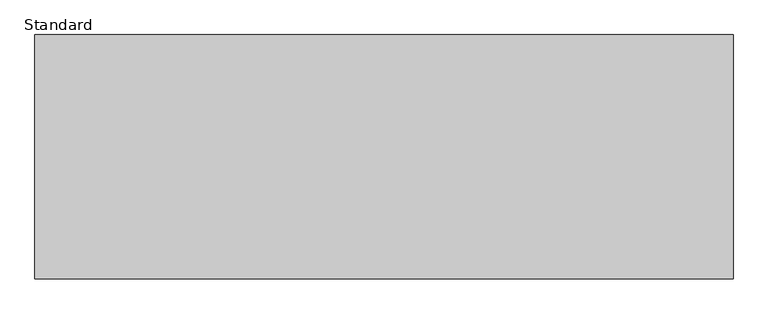
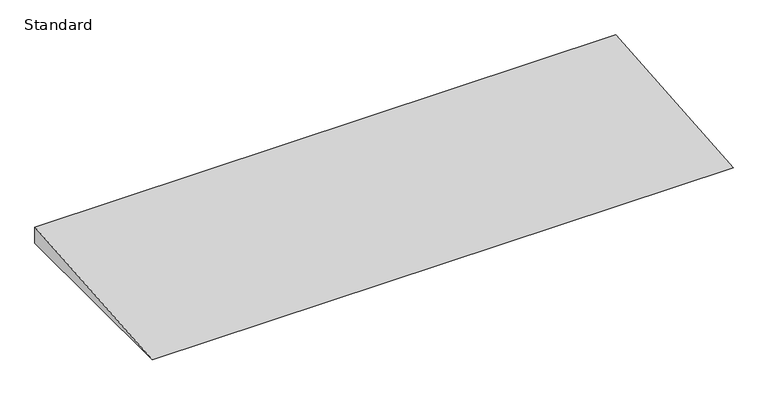
"""IFC4 building model written with IfcOpenShell, lengths in millimetres: ramp geometry, Standard."""

from ifc_helpers import new_model, si_unit, frame, origin, place, context, project, spatial, polyline, outline, extrude, source, transform, mapped, element, save


def standard_ef43e6ca(model_context):
    return source(origin(), model_context, "Body", "SweptSolid", [
        extrude(outline(polyline([(-9586.6553244, 914.4), (-8519.8553244, 1003.3), (-8519.8553244, 914.4), (-9586.6553244, 914.4)])), frame((559.5495839, 0.0, 0.0), z_axis=(1.0, 0.0, 0.0), x_axis=(0.0, 1.0, 0.0)), (0.0, 0.0, 1.0), 3048.0),
    ])


if __name__ == "__main__":
    model = new_model("IFC4")
    model_context = context("Model", 3, world=origin())
    ifc_project = project(units=[si_unit("LENGTHUNIT", "METRE", prefix="MILLI")], contexts=[model_context])
    site = spatial("IfcSite", under=ifc_project)
    building = spatial("IfcBuilding", under=site)
    placement = place(None, origin())
    standard_shape = standard_ef43e6ca(model_context)
    element("IfcRamp", 1, ObjectType="Standard", at=placement, inside=building, context=model_context, shape_type="MappedRepresentation", body=[
        mapped(standard_shape, transform((0.0, 0.0, 0.0), x_axis=(1.0, 0.0, 0.0), y_axis=(0.0, 1.0, 0.0), z_axis=(0.0, 0.0, 1.0))),
    ])
    save(model, "model.ifc")
